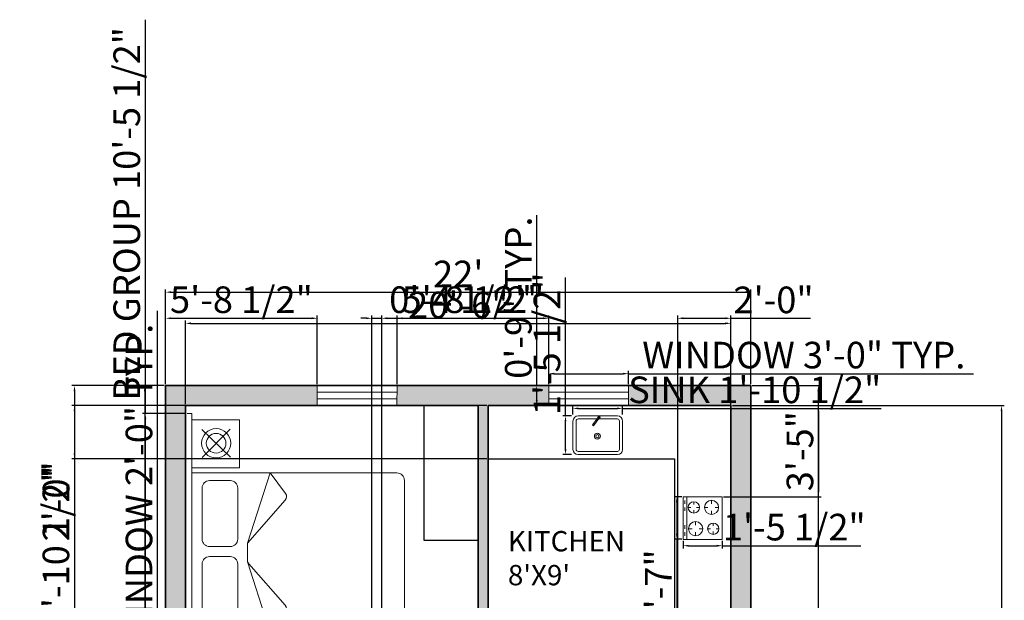
# Model space of a CAD drawing. Units: inches. Extents: x 1810 to 2254, y 313 to 1026.
# Tile 7 of 7: x 1810 to 2254, y 764 to 1026. Entities that reach past the tile are written whole.
import ezdxf

# ---------------------------------------------------------------- set-up
doc = ezdxf.new("R2010")
doc.units = ezdxf.units.IN
for name, color, linetype, lineweight in [('A-ANNO-DIMS', 2, 'Continuous', 18), ('A-AREA-IDEN', 7, 'Continuous', 25), ('A-EQPM', 9, 'Continuous', 18), ('A-FLOR-CASE', 8, 'Continuous', 25), ('A-FLOR-FIXT', 9, 'Continuous', 18), ('A-FURN', 8, 'Continuous', 18), ('A-GLAZ', 4, 'Continuous', 18), ('A-WALL', 7, 'Continuous', 35)]:
    doc.layers.add(name, color=color, linetype=linetype, lineweight=lineweight)
doc.layers.add('A-WALL-PATT', color=252, linetype='Continuous', lineweight=13, true_color=0x939598)
doc.styles.get("Standard").update_dxf_attribs({"font": 'arial.ttf'})
doc.dimstyles.new('ISO-25', dxfattribs={"dimtxt": 12, "dimasz": 2.5, "dimexe": 1.25, "dimexo": 0.625, "dimtad": 1, "dimdec": 1, "dimlunit": 4, "dimtxsty": 'Standard', "dimcen": 2.5, "dimadec": 0, "dimazin": 0, "dimtfac": 1, "dimtdec": 1, "dimtmove": 0, "dimatfit": 3, "dimfxl": 1, "dimarcsym": 0})

# ---------------------------------------------------------------- blocks, each defined once
blk = doc.blocks.new('A$C5C1F5B49')
for p, q in [((0, 2), (0, 2.0434)), ((2.6204, 1.9984), (2.6204, 2.0434)), ((0, 2), (2.6204, 2)), ((0.5102, 2), (0.0602, 2)), ((0.0602, 2), (0.0602, 1.55)), ((0.5102, 1.55), (0.5102, 2)), ((0.5602, 2), (0.5602, 0.07)), ((2.0602, 2), (0.5602, 2)), ((2.0602, 0.07), (2.0602, 2)), ((2.5602, 2), (2.1102, 2)), ((2.1102, 2), (2.1102, 1.55)), ((2.5602, 1.55), (2.5602, 2)), ((0.1574, 1.9028), (0.4225, 1.6377)), ((0.1602, 1.635), (0.4197, 1.9056)), ((1.2033, 1.9024), (0.7221, 1.9024)), ((1.919, 1.9024), (1.4378, 1.9024)), ((2.2074, 1.9028), (2.4725, 1.6377)), ((2.2102, 1.635), (2.4697, 1.9056)), ((0.6521, 1.8324), (0.6521, 1.6369)), ((1.2733, 1.6369), (1.2733, 1.8324)), ((1.3678, 1.8324), (1.3678, 1.6369)), ((1.989, 1.6369), (1.989, 1.8324)), ((0.0602, 1.55), (0.5102, 1.55)), ((0.7221, 1.5669), (1.2033, 1.5669)), ((1.4378, 1.5669), (1.919, 1.5669)), ((2.1102, 1.55), (2.5602, 1.55)), ((0.5602, 1.2611), (1.2132, 1.4737)), ((1.2066, 1.4637), (0.8154, 1.12)), ((1.3997, 1.4761), (1.2396, 1.4761)), ((1.3997, 1.4761), (1.805, 1.12)), ((2.0602, 1.2611), (1.3997, 1.4761)), ((0.7525, 1.1175), (0.5602, 1.2611)), ((1.868, 1.1175), (2.0602, 1.2611)), ((0.6302, 0), (1.9902, 0))]:
    blk.add_line(p, q)
for centre, radius in [((0.2899, 1.7703), 0.1375), ((0.2899, 1.7703), 0.0925), ((2.3399, 1.7703), 0.1375), ((2.3399, 1.7703), 0.0925)]:
    blk.add_circle(centre, radius)
for centre, radius, start, end in [((0.7221, 1.8324), 0.07, 90, 180), ((1.2033, 1.8324), 0.07, 0, 90), ((1.4378, 1.8324), 0.07, 90, 180), ((1.919, 1.8324), 0.07, 0, 90), ((0.7221, 1.6369), 0.07, 180, 270), ((1.2033, 1.6369), 0.07, 270, 0), ((1.4378, 1.6369), 0.07, 180, 270), ((1.919, 1.6369), 0.07, 270, 0), ((1.2396, 1.4261), 0.05, 90, 131.30416), ((1.2287, 1.4261), 0.05, 90, 108.03402), ((0.7824, 1.1575), 0.05, 233.24211, 311.30416), ((1.838, 1.1575), 0.05, 228.69584, 306.75789), ((0.6302, 0.07), 0.07, 180, 270), ((1.9902, 0.07), 0.07, 270, 0)]:
    blk.add_arc(centre, radius, start, end)
blk = doc.blocks.new('A$C5B032A53')
for p, q in [((0, 60), (0, 384)), ((36, 60), (36, 384)), ((60, 444), (509, 444)), ((60, 408), (275, 408)), ((286, 422), (224, 339)), ((224, 339), (236, 331)), ((296, 412), (236, 331)), ((293, 408), (509, 408)), ((533, 384), (533, 60)), ((569, 384), (569, 60)), ((509, 36), (60, 36)), ((509, 0), (60, 0))]:
    blk.add_line(p, q)
for centre, radius in [((299, 426), 13.7), ((299, 426), 7.24), ((280, 211), 34), ((280, 211), 18)]:
    blk.add_circle(centre, radius)
for centre, radius, start, end in [((60, 384), 60, 90, 180), ((60, 384), 24, 90, 180), ((509, 384), 60, 360, 90), ((509, 384), 24, 360, 90), ((60, 60), 60, 180, 270), ((60, 60), 24, 180, 270), ((509, 60), 24, 270, 0), ((509, 60), 60, 270, 0)]:
    blk.add_arc(centre, radius, start, end)
blk = doc.blocks.new('A$C3FB84F07')
at = {"linetype": 'ByBlock'}
for p, q in [((488, 447), (0, 447)), ((0, 447), (0, 0)), ((122, 406), (122, 366)), ((301, 345), (333, 345)), ((366, 410), (366, 378)), ((431, 345), (398, 345)), ((488, 0), (488, 447)), ((41, 325), (81, 325)), ((122, 244), (122, 284)), ((203, 325), (163, 325)), ((366, 280), (366, 313)), ((57, 122), (89, 122)), ((122, 187), (122, 154)), ((187, 122), (154, 122)), ((284, 142), (325, 142)), ((366, 224), (366, 183)), ((447, 142), (406, 142)), ((0, 41), (488, 41)), ((0, 0), (488, 0)), ((41, 20), (81, 20)), ((122, 57), (122, 89)), ((122, 20), (163, 20)), ((325, 20), (366, 20)), ((366, 61), (366, 102)), ((406, 20), (447, 20))]:
    blk.add_line(p, q, dxfattribs=at)
for centre, radius in [((122, 325), 81.3), ((366, 345), 65), ((122, 122), 65), ((366, 142), 81.3)]:
    blk.add_circle(centre, radius, dxfattribs=at)
blk = doc.blocks.new('*D21')
at = {"layer": 'A-ANNO-DIMS', "color": 0, "lineweight": -2, "transparency": 16777216}
for p, q in [((1875.36, 861.24), (1875.36, 904.04)), ((1877.86, 902.79), (2136.86, 902.79)), ((2139.36, 861.24), (2139.36, 904.04))]:
    blk.add_line(p, q, dxfattribs=at)
at = {"layer": 'A-ANNO-DIMS', "color": 0, "transparency": 16777216}
for points in [[(1877.86, 903.21), (1877.86, 902.38), (1875.36, 902.79)], [(2136.86, 903.21), (2136.86, 902.38), (2139.36, 902.79)]]:
    blk.add_solid(points, dxfattribs=at)
at = {"layer": 'Defpoints', "color": 0, "transparency": 16777216}
for p in [(2139.36, 902.79), (1875.36, 860.61), (2139.36, 860.61)]:
    blk.add_point(p, dxfattribs=at)
at = {"layer": 'A-ANNO-DIMS', "color": 0, "transparency": 16777216, "insert": (2007.36, 909.44), "char_height": 12, "attachment_point": 5}
blk.add_mtext("22'", dxfattribs=at)
blk = doc.blocks.new('*D22')
at = {"layer": 'A-ANNO-DIMS', "color": 0, "lineweight": -2, "transparency": 16777216}
for p, q in [((1884.36, 852.24), (1884.36, 889.98)), ((1886.86, 888.73), (2127.86, 888.73)), ((2130.36, 852.24), (2130.36, 889.98))]:
    blk.add_line(p, q, dxfattribs=at)
at = {"layer": 'A-ANNO-DIMS', "color": 0, "transparency": 16777216}
for points in [[(1886.86, 889.15), (1886.86, 888.31), (1884.36, 888.73)], [(2127.86, 889.15), (2127.86, 888.31), (2130.36, 888.73)]]:
    blk.add_solid(points, dxfattribs=at)
at = {"layer": 'Defpoints', "color": 0, "transparency": 16777216}
for p in [(2130.36, 888.73), (1884.36, 851.61), (2130.36, 851.61)]:
    blk.add_point(p, dxfattribs=at)
at = {"layer": 'A-ANNO-DIMS', "color": 0, "transparency": 16777216, "insert": (2007.36, 895.48), "char_height": 12, "attachment_point": 5}
blk.add_mtext('20\'-6"', dxfattribs=at)
blk = doc.blocks.new('*D23')
at = {"layer": 'A-ANNO-DIMS', "color": 0, "lineweight": -2, "transparency": 16777216}
for p, q in [((2130.99, 851.61), (2253.63, 851.61)), ((2252.38, 849.11), (2252.38, 437.11)), ((2130.99, 434.61), (2253.63, 434.61))]:
    blk.add_line(p, q, dxfattribs=at)
at = {"layer": 'A-ANNO-DIMS', "color": 0, "transparency": 16777216}
for points in [[(2251.96, 849.11), (2252.8, 849.11), (2252.38, 851.61)], [(2251.96, 437.11), (2252.8, 437.11), (2252.38, 434.61)]]:
    blk.add_solid(points, dxfattribs=at)
at = {"layer": 'Defpoints', "color": 0, "transparency": 16777216}
for p in [(2130.36, 851.61), (2130.36, 434.61), (2252.38, 434.61)]:
    blk.add_point(p, dxfattribs=at)
at = {"layer": 'A-ANNO-DIMS', "color": 0, "transparency": 16777216, "insert": (2245.62, 643.11), "char_height": 12, "attachment_point": 5, "rotation": 90}
blk.add_mtext('34\'-9"', dxfattribs=at)
blk = doc.blocks.new('*D25')
at = {"layer": 'A-ANNO-DIMS', "color": 0, "lineweight": -2, "transparency": 16777216}
for p, q in [((1874.74, 860.61), (1864.75, 860.61)), ((1866, 858.11), (1866, 483.61)), ((1874.74, 481.11), (1864.75, 481.11))]:
    blk.add_line(p, q, dxfattribs=at)
at = {"layer": 'A-ANNO-DIMS', "color": 0, "transparency": 16777216}
for points in [[(1865.58, 858.11), (1866.42, 858.11), (1866, 860.61)], [(1865.58, 483.61), (1866.42, 483.61), (1866, 481.11)]]:
    blk.add_solid(points, dxfattribs=at)
at = {"layer": 'Defpoints', "color": 0, "transparency": 16777216}
for p in [(1875.36, 860.61), (1866, 481.11), (1875.36, 481.11)]:
    blk.add_point(p, dxfattribs=at)
at = {"layer": 'A-ANNO-DIMS', "color": 0, "transparency": 16777216, "insert": (1851.22, 670.86), "char_height": 12, "attachment_point": 5, "rotation": 90}
blk.add_mtext('31\'-7{\\H1x;\\S1/2;}"', dxfattribs=at)
blk = doc.blocks.new('WIN-36IN-WALL9')
for p, q in [((0, 9), (0, 0)), ((36, 9), (36, 0)), ((0, 6), (36, 6)), ((0, 3), (36, 3))]:
    blk.add_line(p, q)
blk = doc.blocks.new('*D32')
at = {"layer": 'A-ANNO-DIMS', "color": 0, "lineweight": -2, "transparency": 16777216}
for p, q in [((2048.15, 861.24), (2048.15, 867.26)), ((2050.65, 866.01), (2081.65, 866.01)), ((2084.15, 861.24), (2084.15, 867.26)), ((2084.15, 866.01), (2239.75, 866.01))]:
    blk.add_line(p, q, dxfattribs=at)
at = {"layer": 'A-ANNO-DIMS', "color": 0, "transparency": 16777216}
for points in [[(2050.65, 866.43), (2050.65, 865.6), (2048.15, 866.01)], [(2081.65, 866.43), (2081.65, 865.6), (2084.15, 866.01)]]:
    blk.add_solid(points, dxfattribs=at)
at = {"layer": 'Defpoints', "color": 0, "transparency": 16777216}
for p in [(2084.15, 866.01), (2048.15, 860.61), (2084.15, 860.61)]:
    blk.add_point(p, dxfattribs=at)
at = {"layer": 'A-ANNO-DIMS', "color": 0, "transparency": 16777216, "insert": (2163.2, 872.85), "char_height": 12, "attachment_point": 5}
blk.add_mtext('WINDOW 3\'-0" TYP.', dxfattribs=at)
blk = doc.blocks.new('*D33')
at = {"layer": 'A-ANNO-DIMS', "color": 0, "lineweight": -2, "transparency": 16777216}
for p, q in [((2042.75, 860.61), (2042.75, 937.51)), ((2047.53, 860.61), (2041.5, 860.61)), ((2042.75, 854.11), (2042.75, 858.11)), ((2047.53, 851.61), (2041.5, 851.61))]:
    blk.add_line(p, q, dxfattribs=at)
at = {"layer": 'A-ANNO-DIMS', "color": 0, "transparency": 16777216}
for points in [[(2042.34, 858.11), (2043.17, 858.11), (2042.75, 860.61)], [(2042.34, 854.11), (2043.17, 854.11), (2042.75, 851.61)]]:
    blk.add_solid(points, dxfattribs=at)
at = {"layer": 'Defpoints', "color": 0, "transparency": 16777216}
for p in [(2042.75, 860.61), (2048.15, 860.61), (2048.15, 851.61)]:
    blk.add_point(p, dxfattribs=at)
at = {"layer": 'A-ANNO-DIMS', "color": 0, "transparency": 16777216, "insert": (2036, 900.31), "char_height": 12, "attachment_point": 5, "rotation": 90}
blk.add_mtext('0\'-9" TYP.', dxfattribs=at)
blk = doc.blocks.new('*D34')
at = {"layer": 'A-ANNO-DIMS', "color": 0, "lineweight": -2, "transparency": 16777216}
for p, q in [((1871.76, 706.11), (1871.76, 894.3)), ((1874.74, 706.11), (1870.51, 706.11)), ((1871.76, 684.61), (1871.76, 703.61)), ((1874.74, 682.11), (1870.51, 682.11))]:
    blk.add_line(p, q, dxfattribs=at)
at = {"layer": 'A-ANNO-DIMS', "color": 0, "transparency": 16777216}
for points in [[(1871.35, 703.61), (1872.18, 703.61), (1871.76, 706.11)], [(1871.35, 684.61), (1872.18, 684.61), (1871.76, 682.11)]]:
    blk.add_solid(points, dxfattribs=at)
at = {"layer": 'Defpoints', "color": 0, "transparency": 16777216}
for p in [(1871.76, 706.11), (1875.36, 706.11), (1875.36, 682.11)]:
    blk.add_point(p, dxfattribs=at)
at = {"layer": 'A-ANNO-DIMS', "color": 0, "transparency": 16777216, "insert": (1864.93, 801.46), "char_height": 12, "attachment_point": 5, "rotation": 90}
blk.add_mtext('WC WINDOW 2\'-0" TYP.', dxfattribs=at)
blk = doc.blocks.new('*D36')
at = {"layer": 'A-ANNO-DIMS', "color": 0, "lineweight": -2, "transparency": 16777216}
for p, q in [((1866.25, 848.07), (1866.25, 1025.73)), ((1884.47, 848.07), (1865, 848.07)), ((1866.25, 724.95), (1866.25, 845.57)), ((1884.47, 722.45), (1865, 722.45))]:
    blk.add_line(p, q, dxfattribs=at)
at = {"layer": 'A-ANNO-DIMS', "color": 0, "transparency": 16777216}
for points in [[(1865.83, 845.57), (1866.66, 845.57), (1866.25, 848.07)], [(1865.83, 724.95), (1866.66, 724.95), (1866.25, 722.45)]]:
    blk.add_solid(points, dxfattribs=at)
at = {"layer": 'Defpoints', "color": 0, "transparency": 16777216}
for p in [(1866.25, 848.07), (1885.09, 848.07), (1885.09, 722.45)]:
    blk.add_point(p, dxfattribs=at)
at = {"layer": 'A-ANNO-DIMS', "color": 0, "transparency": 16777216, "insert": (1859.41, 938.15), "char_height": 12, "attachment_point": 5, "rotation": 90}
blk.add_mtext('BED GROUP 10\'-5 1/2"', dxfattribs=at)
blk = doc.blocks.new('*D40')
at = {"layer": 'A-ANNO-DIMS', "color": 0, "lineweight": -2, "transparency": 16777216}
for p, q in [((2059.09, 847.61), (2059.09, 851.59)), ((2061.59, 850.34), (2078.98, 850.34)), ((2081.48, 847.61), (2081.48, 851.59)), ((2081.48, 850.34), (2198.14, 850.34))]:
    blk.add_line(p, q, dxfattribs=at)
at = {"layer": 'A-ANNO-DIMS', "color": 0, "transparency": 16777216}
for points in [[(2061.59, 850.76), (2061.59, 849.93), (2059.09, 850.34)], [(2078.98, 850.76), (2078.98, 849.93), (2081.48, 850.34)]]:
    blk.add_solid(points, dxfattribs=at)
at = {"layer": 'Defpoints', "color": 0, "transparency": 16777216}
for p in [(2081.48, 850.34), (2059.09, 846.98), (2081.48, 846.98)]:
    blk.add_point(p, dxfattribs=at)
at = {"layer": 'A-ANNO-DIMS', "color": 0, "transparency": 16777216, "insert": (2141.06, 857.17), "char_height": 12, "attachment_point": 5}
blk.add_mtext('SINK 1\'-10 1/2"', dxfattribs=at)
blk = doc.blocks.new('*D41')
at = {"layer": 'A-ANNO-DIMS', "color": 0, "lineweight": -2, "transparency": 16777216}
for p, q in [((2055.74, 846.98), (2055.74, 909.47)), ((2058.47, 846.98), (2054.49, 846.98)), ((2055.74, 832.02), (2055.74, 844.48)), ((2058.47, 829.52), (2054.49, 829.52))]:
    blk.add_line(p, q, dxfattribs=at)
at = {"layer": 'A-ANNO-DIMS', "color": 0, "transparency": 16777216}
for points in [[(2055.32, 844.48), (2056.15, 844.48), (2055.74, 846.98)], [(2055.32, 832.02), (2056.15, 832.02), (2055.74, 829.52)]]:
    blk.add_solid(points, dxfattribs=at)
at = {"layer": 'Defpoints', "color": 0, "transparency": 16777216}
for p in [(2055.74, 846.98), (2059.09, 846.98), (2059.09, 829.52)]:
    blk.add_point(p, dxfattribs=at)
at = {"layer": 'A-ANNO-DIMS', "color": 0, "transparency": 16777216, "insert": (2048.91, 879.48), "char_height": 12, "attachment_point": 5, "rotation": 90}
blk.add_mtext('1\'-5 1/2"', dxfattribs=at)
blk = doc.blocks.new('*D42')
at = {"layer": 'A-ANNO-DIMS', "color": 0, "lineweight": -2, "transparency": 16777216}
for p, q in [((2108.19, 810.48), (2104.68, 810.48)), ((2105.93, 807.98), (2105.93, 793.78)), ((2108.19, 791.28), (2104.68, 791.28)), ((2105.93, 791.28), (2105.93, 667.28))]:
    blk.add_line(p, q, dxfattribs=at)
at = {"layer": 'A-ANNO-DIMS', "color": 0, "transparency": 16777216}
for points in [[(2105.52, 807.98), (2106.35, 807.98), (2105.93, 810.48)], [(2105.52, 793.78), (2106.35, 793.78), (2105.93, 791.28)]]:
    blk.add_solid(points, dxfattribs=at)
at = {"layer": 'Defpoints', "color": 0, "transparency": 16777216}
for p in [(2108.81, 810.48), (2105.93, 791.28), (2108.81, 791.28)]:
    blk.add_point(p, dxfattribs=at)
at = {"layer": 'A-ANNO-DIMS', "color": 0, "transparency": 16777216, "insert": (2099.1, 728.03), "char_height": 12, "attachment_point": 5, "rotation": 90}
blk.add_mtext('COOKTOP 1\'-7"', dxfattribs=at)
blk = doc.blocks.new('*D43')
at = {"layer": 'A-ANNO-DIMS', "color": 0, "lineweight": -2, "transparency": 16777216}
for p, q in [((2108.81, 790.65), (2108.81, 787.15)), ((2126.41, 790.65), (2126.41, 787.15)), ((2111.31, 788.4), (2123.91, 788.4)), ((2126.41, 788.4), (2188.89, 788.4))]:
    blk.add_line(p, q, dxfattribs=at)
at = {"layer": 'A-ANNO-DIMS', "color": 0, "transparency": 16777216}
for points in [[(2111.31, 788.81), (2111.31, 787.98), (2108.81, 788.4)], [(2123.91, 788.81), (2123.91, 787.98), (2126.41, 788.4)]]:
    blk.add_solid(points, dxfattribs=at)
at = {"layer": 'Defpoints', "color": 0, "transparency": 16777216}
for p in [(2108.81, 791.28), (2126.41, 791.28), (2126.41, 788.4)]:
    blk.add_point(p, dxfattribs=at)
at = {"layer": 'A-ANNO-DIMS', "color": 0, "transparency": 16777216, "insert": (2158.9, 795.23), "char_height": 12, "attachment_point": 5}
blk.add_mtext('1\'-5 1/2"', dxfattribs=at)
blk = doc.blocks.new('*D50')
at = {"layer": 'A-ANNO-DIMS', "color": 0, "lineweight": -2, "transparency": 16777216}
for p, q in [((2139.99, 860.61), (2171.01, 860.61)), ((2169.76, 359.11), (2169.76, 858.11)), ((2139.99, 356.61), (2171.01, 356.61))]:
    blk.add_line(p, q, dxfattribs=at)
at = {"layer": 'A-ANNO-DIMS', "color": 0, "transparency": 16777216}
for points in [[(2169.35, 858.11), (2170.18, 858.11), (2169.76, 860.61)], [(2169.35, 359.11), (2170.18, 359.11), (2169.76, 356.61)]]:
    blk.add_solid(points, dxfattribs=at)
at = {"layer": 'Defpoints', "color": 0, "transparency": 16777216}
for p in [(2139.36, 860.61), (2169.76, 860.61), (2139.36, 356.61)]:
    blk.add_point(p, dxfattribs=at)
at = {"layer": 'A-ANNO-DIMS', "color": 0, "transparency": 16777216, "insert": (2163.01, 608.61), "char_height": 12, "attachment_point": 5, "rotation": 90}
blk.add_mtext('42\'-0"', dxfattribs=at)
blk = doc.blocks.new('*D51')
at = {"layer": 'A-ANNO-DIMS', "color": 0, "lineweight": -2, "transparency": 16777216}
for p, q in [((1875.36, 861.24), (1875.36, 892.26)), ((1877.86, 891.01), (1941.28, 891.01)), ((1943.78, 861.24), (1943.78, 892.26))]:
    blk.add_line(p, q, dxfattribs=at)
at = {"layer": 'A-ANNO-DIMS', "color": 0, "transparency": 16777216}
for points in [[(1877.86, 891.43), (1877.86, 890.6), (1875.36, 891.01)], [(1941.28, 891.43), (1941.28, 890.6), (1943.78, 891.01)]]:
    blk.add_solid(points, dxfattribs=at)
at = {"layer": 'Defpoints', "color": 0, "transparency": 16777216}
for p in [(1943.78, 891.01), (1875.36, 860.61), (1943.78, 860.61)]:
    blk.add_point(p, dxfattribs=at)
at = {"layer": 'A-ANNO-DIMS', "color": 0, "transparency": 16777216, "insert": (1909.57, 897.84), "char_height": 12, "attachment_point": 5}
blk.add_mtext('5\'-8 1/2"', dxfattribs=at)
blk = doc.blocks.new('*D52')
at = {"layer": 'A-ANNO-DIMS', "color": 0, "lineweight": -2, "transparency": 16777216}
for p, q in [((1979.78, 861.24), (1979.78, 892.26)), ((1982.28, 891.01), (2045.65, 891.01)), ((2048.15, 861.24), (2048.15, 892.26))]:
    blk.add_line(p, q, dxfattribs=at)
at = {"layer": 'A-ANNO-DIMS', "color": 0, "transparency": 16777216}
for points in [[(1982.28, 891.43), (1982.28, 890.6), (1979.78, 891.01)], [(2045.65, 891.43), (2045.65, 890.6), (2048.15, 891.01)]]:
    blk.add_solid(points, dxfattribs=at)
at = {"layer": 'Defpoints', "color": 0, "transparency": 16777216}
for p in [(2048.15, 891.01), (1979.78, 860.61), (2048.15, 860.61)]:
    blk.add_point(p, dxfattribs=at)
at = {"layer": 'A-ANNO-DIMS', "color": 0, "transparency": 16777216, "insert": (2013.97, 897.84), "char_height": 12, "attachment_point": 5}
blk.add_mtext('5\'-8 1/2"', dxfattribs=at)
blk = doc.blocks.new('*D55')
at = {"layer": 'A-ANNO-DIMS', "color": 0, "lineweight": -2, "transparency": 16777216}
for p, q in [((1874.74, 860.61), (1833.05, 860.61)), ((1834.3, 858.11), (1834.3, 708.61)), ((1874.74, 706.11), (1833.05, 706.11))]:
    blk.add_line(p, q, dxfattribs=at)
at = {"layer": 'A-ANNO-DIMS', "color": 0, "transparency": 16777216}
for points in [[(1833.89, 858.11), (1834.72, 858.11), (1834.3, 860.61)], [(1833.89, 708.61), (1834.72, 708.61), (1834.3, 706.11)]]:
    blk.add_solid(points, dxfattribs=at)
at = {"layer": 'Defpoints', "color": 0, "transparency": 16777216}
for p in [(1875.36, 860.61), (1834.3, 706.11), (1875.36, 706.11)]:
    blk.add_point(p, dxfattribs=at)
at = {"layer": 'A-ANNO-DIMS', "color": 0, "transparency": 16777216, "insert": (1827.47, 783.36), "char_height": 12, "attachment_point": 5, "rotation": 90}
blk.add_mtext('12\'-10 1/2"', dxfattribs=at)
blk = doc.blocks.new('*D58')
at = {"layer": 'A-ANNO-DIMS', "color": 0, "lineweight": -2, "transparency": 16777216}
for p, q in [((2020.24, 851.61), (1833.05, 851.61)), ((1834.3, 849.11), (1834.3, 830.11)), ((2020.24, 827.61), (1833.05, 827.61)), ((1834.3, 827.61), (1834.3, 791.76))]:
    blk.add_line(p, q, dxfattribs=at)
at = {"layer": 'A-ANNO-DIMS', "color": 0, "transparency": 16777216}
for points in [[(1833.89, 849.11), (1834.72, 849.11), (1834.3, 851.61)], [(1833.89, 830.11), (1834.72, 830.11), (1834.3, 827.61)]]:
    blk.add_solid(points, dxfattribs=at)
at = {"layer": 'Defpoints', "color": 0, "transparency": 16777216}
for p in [(2020.86, 851.61), (1834.3, 827.61), (2020.86, 827.61)]:
    blk.add_point(p, dxfattribs=at)
at = {"layer": 'A-ANNO-DIMS', "color": 0, "transparency": 16777216, "insert": (1827.55, 808.43), "char_height": 12, "attachment_point": 5, "rotation": 90}
blk.add_mtext('2\'-0"', dxfattribs=at)
blk = doc.blocks.new('*D61')
at = {"layer": 'A-ANNO-DIMS', "color": 0, "lineweight": -2, "transparency": 16777216}
for p, q in [((2106.36, 559.74), (2106.36, 892.26)), ((2108.86, 891.01), (2127.86, 891.01)), ((2130.36, 559.74), (2130.36, 892.26)), ((2130.36, 891.01), (2166.22, 891.01))]:
    blk.add_line(p, q, dxfattribs=at)
at = {"layer": 'A-ANNO-DIMS', "color": 0, "transparency": 16777216}
for points in [[(2108.86, 891.43), (2108.86, 890.6), (2106.36, 891.01)], [(2127.86, 891.43), (2127.86, 890.6), (2130.36, 891.01)]]:
    blk.add_solid(points, dxfattribs=at)
at = {"layer": 'Defpoints', "color": 0, "transparency": 16777216}
for p in [(2130.36, 891.01), (2106.36, 559.11), (2130.36, 559.11)]:
    blk.add_point(p, dxfattribs=at)
at = {"layer": 'A-ANNO-DIMS', "color": 0, "transparency": 16777216, "insert": (2149.54, 897.76), "char_height": 12, "attachment_point": 5}
blk.add_mtext('2\'-0"', dxfattribs=at)
blk = doc.blocks.new('*D65')
at = {"layer": 'A-ANNO-DIMS', "color": 0, "lineweight": -2, "transparency": 16777216}
for p, q in [((1965.86, 891.01), (1963.36, 891.01)), ((1968.36, 679.98), (1968.36, 892.26)), ((1968.36, 891.01), (1972.86, 891.01)), ((1972.86, 679.98), (1972.86, 892.26)), ((1975.36, 891.01), (2038.97, 891.01))]:
    blk.add_line(p, q, dxfattribs=at)
at = {"layer": 'A-ANNO-DIMS', "color": 0, "transparency": 16777216}
for points in [[(1965.86, 891.43), (1965.86, 890.6), (1968.36, 891.01)], [(1975.36, 891.43), (1975.36, 890.6), (1972.86, 891.01)]]:
    blk.add_solid(points, dxfattribs=at)
at = {"layer": 'Defpoints', "color": 0, "transparency": 16777216}
for p in [(1972.86, 891.01), (1968.36, 679.36), (1972.86, 679.36)]:
    blk.add_point(p, dxfattribs=at)
at = {"layer": 'A-ANNO-DIMS', "color": 0, "transparency": 16777216, "insert": (2008.42, 897.84), "char_height": 12, "attachment_point": 5}
blk.add_mtext('0\'-4 1/2"', dxfattribs=at)
blk = doc.blocks.new('*D68')
at = {"layer": 'A-ANNO-DIMS', "color": 0, "lineweight": -2, "transparency": 16777216}
for p, q in [((2020.86, 826.99), (2020.86, 323.71)), ((2104.86, 826.99), (2104.86, 323.71)), ((2023.36, 324.96), (2102.36, 324.96))]:
    blk.add_line(p, q, dxfattribs=at)
at = {"layer": 'A-ANNO-DIMS', "color": 0, "transparency": 16777216}
for points in [[(2023.36, 325.38), (2023.36, 324.55), (2020.86, 324.96)], [(2102.36, 325.38), (2102.36, 324.55), (2104.86, 324.96)]]:
    blk.add_solid(points, dxfattribs=at)
at = {"layer": 'Defpoints', "color": 0, "transparency": 16777216}
for p in [(2020.86, 827.61), (2104.86, 827.61), (2104.86, 324.96)]:
    blk.add_point(p, dxfattribs=at)
at = {"layer": 'A-ANNO-DIMS', "color": 0, "transparency": 16777216, "insert": (2062.86, 331.72), "char_height": 12, "attachment_point": 5}
blk.add_mtext('7\'-0"', dxfattribs=at)
blk = doc.blocks.new('*D69')
at = {"layer": 'A-ANNO-DIMS', "color": 0, "lineweight": -2, "transparency": 16777216}
for p, q in [((2130.99, 851.61), (2171.01, 851.61)), ((2169.76, 849.11), (2169.76, 812.98)), ((2127.04, 810.48), (2171.01, 810.48))]:
    blk.add_line(p, q, dxfattribs=at)
at = {"layer": 'A-ANNO-DIMS', "color": 0, "transparency": 16777216}
for points in [[(2169.35, 849.11), (2170.18, 849.11), (2169.76, 851.61)], [(2169.35, 812.98), (2170.18, 812.98), (2169.76, 810.48)]]:
    blk.add_solid(points, dxfattribs=at)
at = {"layer": 'Defpoints', "color": 0, "transparency": 16777216}
for p in [(2130.36, 851.61), (2126.41, 810.48), (2169.76, 810.48)]:
    blk.add_point(p, dxfattribs=at)
at = {"layer": 'A-ANNO-DIMS', "color": 0, "transparency": 16777216, "insert": (2163.01, 831.04), "char_height": 12, "attachment_point": 5, "rotation": 90}
blk.add_mtext('3\'-5"', dxfattribs=at)

msp = doc.modelspace()

# ---------------------------------------------------------------- hatches: boundary and pattern name
at = {"layer": 'A-WALL-PATT'}
h = msp.add_hatch(color=256, dxfattribs=at)
h.dxf.hatch_style = 1
h.paths.add_polyline_path([(1943.78, 860.61), (1875.36, 860.61), (1875.36, 706.11), (1884.36, 706.11), (1884.36, 715.11), (1968.36, 715.11), (1968.36, 703.36), (1971.96, 703.36), (1972.86, 703.36), (1972.86, 715.11), (1976.68, 715.11), (1976.68, 719.61), (1884.36, 719.61), (1884.36, 851.61), (1943.73, 851.61)])
h.paths.add_polyline_path([(2048.15, 860.61), (1979.78, 860.61), (1979.73, 851.61), (2016.36, 851.61), (2016.36, 719.61), (2012.68, 719.61), (2012.68, 716.01), (2012.68, 715.11), (2024.44, 715.11), (2024.44, 719.61), (2020.86, 719.61), (2020.86, 851.61), (2048.15, 851.61)])
h.paths.add_polyline_path([(2139.36, 860.61), (2084.15, 860.61), (2084.15, 851.61), (2130.36, 851.61), (2130.36, 719.61), (2060.44, 719.61), (2060.44, 716.01), (2060.44, 715.11), (2130.36, 715.11), (2130.36, 673.52), (2139.36, 673.52)])
h.paths.add_polyline_path([(1884.36, 682.11), (1875.36, 682.11), (1875.36, 654.79), (1884.36, 654.79), (1884.36, 662.61), (1968.36, 662.61), (1968.36, 647.42), (1971.96, 647.42), (1972.86, 647.42), (1972.86, 679.36), (1968.36, 679.36), (1968.36, 667.11), (1884.36, 667.11)])
h.paths.add_polyline_path([(1884.36, 610.11), (1972.86, 610.11), (1976.27, 610.11), (1976.27, 614.61), (1972.86, 614.61), (1972.86, 623.42), (1968.36, 623.42), (1968.36, 614.61), (1884.36, 614.61), (1884.36, 630.79), (1875.36, 630.79), (1875.36, 481.11), (1939.68, 481.11), (1939.68, 490.11), (1884.36, 490.11)])
h.paths.add_polyline_path([(2007.36, 518.61), (2038.86, 518.61), (2038.86, 494.59), (2043.36, 494.59), (2043.36, 518.61), (2070.36, 518.61), (2070.36, 523.11), (2007.36, 523.11), (2007.36, 614.61), (2000.27, 614.61), (2000.27, 610.11), (2003.36, 610.11), (2003.36, 490.11), (1975.68, 490.11), (1975.68, 481.11), (2007.36, 481.11)])
h.paths.add_polyline_path([(2139.36, 637.52), (2130.36, 637.52), (2130.36, 434.61), (2043.36, 434.61), (2043.36, 458.59), (2038.86, 458.59), (2038.86, 434.61), (2035.41, 434.61), (2035.41, 431.01), (2035.41, 425.61), (2139.36, 425.61)])

# ---------------------------------------------------------------- linework, layer by layer
at = {"layer": 'A-FLOR-CASE'}
for p, q in [((2016.36, 851.61), (1991.9, 851.61)), ((1991.9, 851.61), (1991.9, 790.95)), ((2020.86, 827.61), (2104.86, 827.61)), ((2104.86, 827.61), (2104.86, 719.61)), ((1991.9, 790.95), (2016.36, 790.95))]:
    msp.add_line(p, q, dxfattribs=at)
at = {"layer": 'A-GLAZ'}
for p, q in [((1943.73, 851.61), (1943.78, 860.61)), ((1943.76, 857.61), (1979.76, 857.61)), ((1979.73, 851.61), (1979.78, 860.61)), ((1943.75, 854.61), (1979.75, 854.61))]:
    msp.add_line(p, q, dxfattribs=at)
at = {"layer": 'A-WALL'}
for p, q in [((1875.36, 860.61), (2139.36, 860.61)), ((1875.36, 860.61), (1875.36, 481.11)), ((2139.36, 860.61), (2139.36, 425.61)), ((1884.36, 851.61), (2016.36, 851.61)), ((1884.36, 851.61), (1884.36, 719.61)), ((2016.36, 851.61), (2016.36, 719.61)), ((2020.86, 851.61), (2020.86, 719.61)), ((2020.86, 851.61), (2130.36, 851.61)), ((2130.36, 851.61), (2130.36, 719.61))]:
    msp.add_line(p, q, dxfattribs=at)

# ---------------------------------------------------------------- block references
at = {"layer": 'A-EQPM', "xscale": 0.0393700787401575, "yscale": 0.0393700787401575, "zscale": 0.0393700787401575, "rotation": 270}
msp.add_blockref('A$C3FB84F07', (2108.81, 810.48), dxfattribs=at)
at = {"layer": 'A-FLOR-FIXT', "xscale": 0.0393700787401575, "yscale": 0.0393700787401575, "zscale": 0.0393700787401575}
msp.add_blockref('A$C5B032A53', (2059.09, 829.52), dxfattribs=at)
at = {"layer": 'A-FURN', "xscale": 47.93842186149659, "yscale": 47.93842186149659, "zscale": 47.93842186149659, "rotation": 90}
msp.add_blockref('A$C5C1F5B49', (1983.05, 722.45), dxfattribs=at)
at = {"layer": 'A-GLAZ'}
msp.add_blockref('WIN-36IN-WALL9', (2048.15, 851.61), dxfattribs=at)

# ---------------------------------------------------------------- texts
at = {"layer": 'A-AREA-IDEN', "insert": (2029.76, 795.02), "char_height": 9.181, "attachment_point": 1}
msp.add_mtext_dynamic_manual_height_columns("KITCHEN\\P8'X9'", width=91.1081, gutter_width=45.91, heights=[0], dxfattribs=at)

# ---------------------------------------------------------------- dimensions: what is measured, and where the dimension line sits
at = {"layer": 'A-ANNO-DIMS'}
for base, p1, p2, angle, text, picture, middle in [((1866.25, 848.07), (1885.09, 722.45), (1885.09, 848.07), 90, 'BED GROUP <>', '*D36', (1859.41, 938.15)), ((2042.75, 860.61), (2048.15, 851.61), (2048.15, 860.61), 90, '<> TYP.', '*D33', (2036, 900.31)), ((1871.76, 706.11), (1875.36, 682.11), (1875.36, 706.11), 90, 'WC WINDOW <> TYP.', '*D34', (1864.93, 801.46)), ((2105.93, 791.28), (2108.81, 810.48), (2108.81, 791.28), 270, 'COOKTOP <>', '*D42', (2099.1, 728.03))]:
    dim = msp.add_linear_dim(base=base, p1=p1, p2=p2, angle=angle, text=text, dimstyle='ISO-25', override={"dimdec": 1, "dimlfac": 1, "dimrnd": 0, "dimzin": 1, "dimdsep": 46, "dimlunit": 4, "dimfrac": 2}, dxfattribs=at)
    dim.commit()
    dim.dimension.update_dxf_attribs({"geometry": picture, "text_midpoint": middle})
for base, p1, p2, override, picture, middle in [((2139.36, 902.79), (1875.36, 860.61), (2139.36, 860.61), {"dimclrd": 0, "dimclre": 0, "dimclrt": 0}, '*D21', (2007.36, 909.44)), ((1943.78, 891.01), (1875.36, 860.61), (1943.78, 860.61), {"dimdec": 1, "dimlfac": 1, "dimrnd": 0, "dimzin": 1, "dimdsep": 46, "dimlunit": 4, "dimfrac": 2}, '*D51', (1909.57, 897.84)), ((1972.86, 891.01), (1968.36, 679.36), (1972.86, 679.36), {"dimdec": 1, "dimlfac": 1, "dimrnd": 0, "dimzin": 1, "dimdsep": 46, "dimlunit": 4, "dimfrac": 2}, '*D65', (2008.42, 897.84)), ((2048.15, 891.01), (1979.78, 860.61), (2048.15, 860.61), {"dimdec": 1, "dimlfac": 1, "dimrnd": 0, "dimzin": 1, "dimdsep": 46, "dimlunit": 4, "dimfrac": 2}, '*D52', (2013.97, 897.84)), ((2130.36, 891.01), (2106.36, 559.11), (2130.36, 559.11), {"dimdec": 1, "dimlfac": 1, "dimrnd": 0, "dimzin": 1, "dimdsep": 46, "dimlunit": 4, "dimfrac": 2}, '*D61', (2149.54, 897.76)), ((2130.36, 888.73), (1884.36, 851.61), (2130.36, 851.61), {"dimclrd": 0, "dimclre": 0, "dimclrt": 0}, '*D22', (2007.36, 895.48)), ((2104.86, 324.96), (2020.86, 827.61), (2104.86, 827.61), {"dimdec": 1, "dimlfac": 1, "dimrnd": 0, "dimzin": 1, "dimdsep": 46, "dimlunit": 4, "dimfrac": 2}, '*D68', (2062.86, 331.72)), ((2126.41, 788.4), (2108.81, 791.28), (2126.41, 791.28), {"dimdec": 1, "dimlfac": 1, "dimrnd": 0, "dimzin": 1, "dimdsep": 46, "dimlunit": 4, "dimfrac": 2}, '*D43', (2158.9, 795.23))]:
    dim = msp.add_linear_dim(base=base, p1=p1, p2=p2, dimstyle='ISO-25', override=override, dxfattribs=at)
    dim.commit()
    dim.dimension.update_dxf_attribs({"geometry": picture, "text_midpoint": middle})
for base, p1, p2, override, picture, middle in [((2055.74, 846.98), (2059.09, 829.52), (2059.09, 846.98), {"dimdec": 1, "dimlfac": 1, "dimrnd": 0, "dimzin": 1, "dimdsep": 46, "dimlunit": 4, "dimfrac": 2}, '*D41', (2048.91, 879.48)), ((1834.3, 706.11), (1875.36, 860.61), (1875.36, 706.11), {"dimdec": 1, "dimlfac": 1, "dimrnd": 0, "dimzin": 1, "dimdsep": 46, "dimlunit": 4, "dimfrac": 2}, '*D55', (1827.47, 783.36)), ((1866, 481.11), (1875.36, 860.61), (1875.36, 481.11), {"dimclrd": 0, "dimclre": 0, "dimclrt": 0}, '*D25', (1851.22, 670.86)), ((2169.76, 860.61), (2139.36, 356.61), (2139.36, 860.61), {"dimdec": 1, "dimlfac": 1, "dimrnd": 0, "dimzin": 1, "dimdsep": 46, "dimlunit": 4, "dimfrac": 2}, '*D50', (2163.01, 608.61)), ((1834.3, 827.61), (2020.86, 851.61), (2020.86, 827.61), {"dimdec": 1, "dimlfac": 1, "dimrnd": 0, "dimzin": 1, "dimdsep": 46, "dimlunit": 4, "dimfrac": 2}, '*D58', (1827.55, 808.43)), ((2169.76, 810.48), (2130.36, 851.61), (2126.41, 810.48), {"dimdec": 1, "dimlfac": 1, "dimrnd": 0, "dimzin": 1, "dimdsep": 46, "dimlunit": 4, "dimfrac": 2}, '*D69', (2163.01, 831.04)), ((2252.38, 434.61), (2130.36, 851.61), (2130.36, 434.61), {"dimclrd": 0, "dimclre": 0, "dimclrt": 0}, '*D23', (2245.62, 643.11))]:
    dim = msp.add_linear_dim(base=base, p1=p1, p2=p2, angle=90, dimstyle='ISO-25', override=override, dxfattribs=at)
    dim.commit()
    dim.dimension.update_dxf_attribs({"geometry": picture, "text_midpoint": middle})
for base, p1, p2, text, picture, middle in [((2084.15, 866.01), (2048.15, 860.61), (2084.15, 860.61), 'WINDOW <> TYP.', '*D32', (2163.2, 872.85)), ((2081.48, 850.34), (2059.09, 846.98), (2081.48, 846.98), 'SINK <>', '*D40', (2141.06, 857.17))]:
    dim = msp.add_linear_dim(base=base, p1=p1, p2=p2, text=text, dimstyle='ISO-25', override={"dimdec": 1, "dimlfac": 1, "dimrnd": 0, "dimzin": 1, "dimdsep": 46, "dimlunit": 4, "dimfrac": 2}, dxfattribs=at)
    dim.commit()
    dim.dimension.update_dxf_attribs({"geometry": picture, "text_midpoint": middle})

doc.saveas('drawing.dxf')
